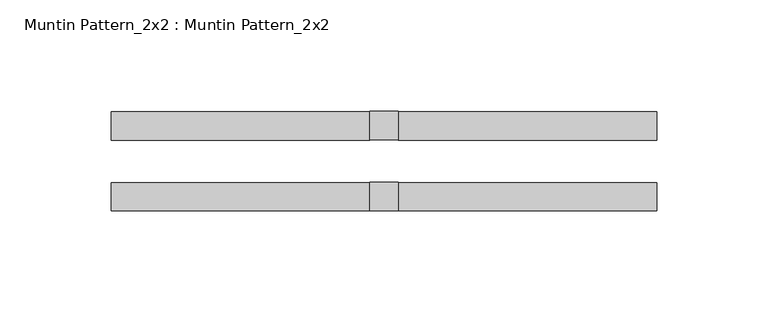
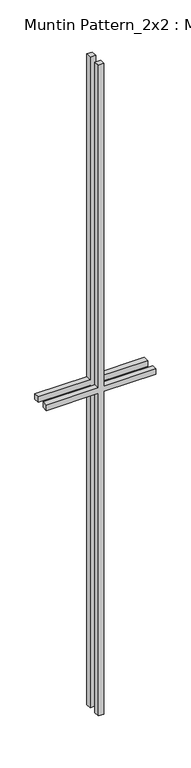
"""IFC4 building model written with IfcOpenShell, lengths in millimetres: proxy geometry, Muntin Pattern_2x2 : Muntin Pattern_2x2."""

from ifc_helpers import new_model, si_unit, frame, origin, place, context, project, spatial, polyline, outline, extrude, source, transform, mapped, element, save


def muntin_pattern_2x2_muntin_pattern_2x2_1c12c043(model_context):
    return source(origin(), model_context, "Body", "SweptSolid", [
        extrude(outline(polyline([(774.7, -6.35), (774.7, -122.2375), (762.0, -122.2375), (762.0, -6.35), (0.0, -6.35), (0.0, 6.35), (762.0, 6.35), (762.0, 122.2375), (774.7, 122.2375), (774.7, 6.35), (1536.7, 6.35), (1536.7, -6.35), (774.7, -6.35)])), frame((0.0, 9.525, 0.0), z_axis=(0.0, 1.0, 0.0), x_axis=(0.0, 0.0, 1.0)), (0.0, 0.0, 1.0), 12.7),
        extrude(outline(polyline([(774.7, -6.35), (774.7, -122.2375), (762.0, -122.2375), (762.0, -6.35), (0.0, -6.35), (0.0, 6.35), (762.0, 6.35), (762.0, 122.2375), (774.7, 122.2375), (774.7, 6.35), (1536.7, 6.35), (1536.7, -6.35), (774.7, -6.35)])), frame((0.0, -22.225, 0.0), z_axis=(0.0, 1.0, 0.0), x_axis=(0.0, 0.0, 1.0)), (0.0, 0.0, 1.0), 12.7),
    ])


if __name__ == "__main__":
    model = new_model("IFC4")
    model_context = context("Model", 3, world=origin())
    ifc_project = project(units=[si_unit("LENGTHUNIT", "METRE", prefix="MILLI")], contexts=[model_context])
    site = spatial("IfcSite", under=ifc_project)
    building = spatial("IfcBuilding", under=site)
    placement = place(None, origin())
    muntin_pattern_2x2_muntin_pattern_2x2_shape = muntin_pattern_2x2_muntin_pattern_2x2_1c12c043(model_context)
    element("IfcBuildingElementProxy", 1, Name="Muntin Pattern_2x2 : Muntin Pattern_2x2", ObjectType="Muntin Pattern_2x2 : Muntin Pattern_2x2", at=placement, inside=building, context=model_context, shape_type="MappedRepresentation", body=[
        mapped(muntin_pattern_2x2_muntin_pattern_2x2_shape, transform((0.0, 0.0, 0.0), x_axis=(1.0, 0.0, 0.0), y_axis=(0.0, 1.0, 0.0), z_axis=(0.0, 0.0, 1.0))),
    ])
    save(model, "model.ifc")

# Revit data of these elements
# Type "Muntin Pattern_2x2 : Muntin Pattern_2x2"
#   Width [instance default] = 4' - 0"
#   Thickness = 0' - 0 1/2"
#   Height [instance default] = 4' - 0"
#   Distance = 0' - 0 3/4"
#   Interior Material [instance default] = none
#   Exterior Material [instance default] = none
#   Default Elevation = 0
# Element 1 (IfcBuildingElementProxy, "Muntin Pattern_2x2 : Muntin Pattern_2x2")
#   Width = 0' - 9 5/8"
#   Height = 5' - 0 1/2"
#   Interior Material = Wood - Stained
#   Exterior Material = Clad - White
#   Materials on its faces: "Clad - White", "Wood - Stained"
# Materials
#   "Clad - White": class "Wood", colour RGB 242 242 238, transparency 0, Cost = 0
#   "Wood - Stained": class "Wood", colour RGB 224 178 126, transparency 0, Cost = 0
